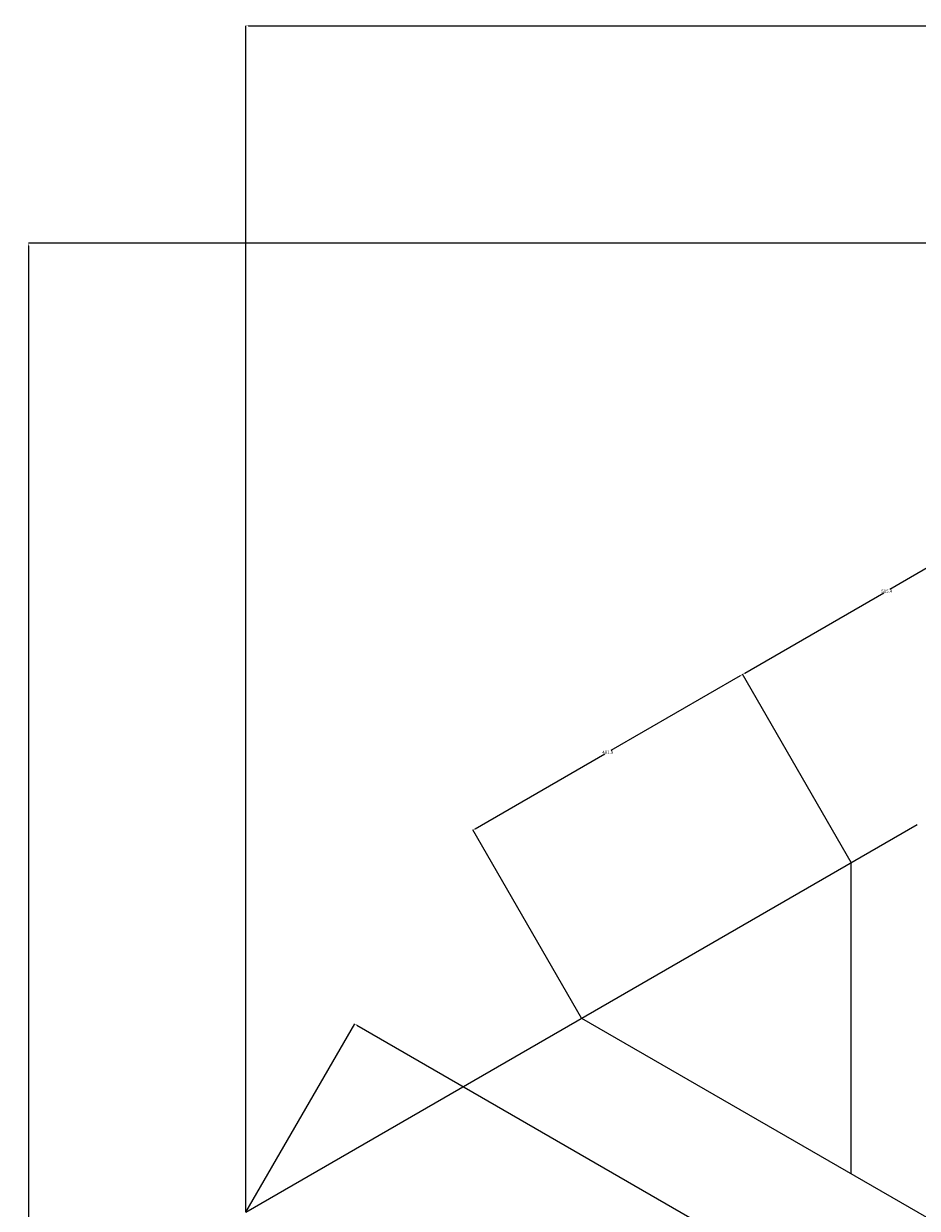
# Model space of a CAD drawing. Units: metres. Extents: x -2391 to 4922, y -635 to 4845.
# Tile 19 of 37: x -2391 to -1008, y 3011 to 4845. Entities that reach past the tile are written whole.
import ezdxf

# ---------------------------------------------------------------- set-up
doc = ezdxf.new("R2010")
doc.units = ezdxf.units.M
doc.header["$MEASUREMENT"] = 0
doc.layers.add('A-ANNO-DIMS', color=2, linetype='Continuous', lineweight=18)
doc.layers.add('A-FLOR-FIXT', color=3, linetype='Continuous', lineweight=25)
doc.styles.get("Standard").update_dxf_attribs({"font": 'arial.ttf'})
doc.dimstyles.get("Standard").update_dxf_attribs({"dimtxt": 5, "dimasz": 4, "dimexe": 0.18, "dimexo": 0.0625, "dimgap": 0.09, "dimtad": 0, "dimtih": 1, "dimtoh": 1, "dimdec": 0, "dimzin": 0, "dimdsep": 46, "dimtxsty": 'Standard', "dimcen": 0.09, "dimadec": 0, "dimazin": 0, "dimtfac": 1, "dimtdec": 0, "dimtofl": 0, "dimtmove": 0, "dimatfit": 3, "dimfxl": 1, "dimtolj": 1, "dimtzin": 0, "dimarcsym": 0})

# ---------------------------------------------------------------- blocks, each defined once
blk = doc.blocks.new('*D9')
at = {"layer": 'A-ANNO-DIMS', "color": 0, "lineweight": -2, "transparency": 16777216}
for p, q in [((-2047.3, 3005.3), (-2047.3, 4842)), ((-2043.3, 4841.8), (-755.9, 4841.8)), ((546.7, 4841.8), (-740.7, 4841.8)), ((550.7, 4505.3), (550.7, 4842))]:
    blk.add_line(p, q, dxfattribs=at)
at = {"layer": 'A-ANNO-DIMS', "color": 0, "transparency": 16777216}
for points in [[(-2043.3, 4842.4), (-2043.3, 4841.1), (-2047.3, 4841.8)], [(546.7, 4842.4), (546.7, 4841.1), (550.7, 4841.8)]]:
    blk.add_solid(points, dxfattribs=at)
at = {"layer": 'Defpoints', "color": 0, "transparency": 16777216}
for p in [(550.7, 4841.8), (550.7, 4505.3), (-2047.3, 3005.3)]:
    blk.add_point(p, dxfattribs=at)
at = {"layer": 'A-ANNO-DIMS', "color": 0, "transparency": 16777216, "insert": (-748.3, 4841.8), "char_height": 5, "attachment_point": 5}
blk.add_mtext('\\A1;2598', dxfattribs=at)
blk = doc.blocks.new('*D10')
at = {"layer": 'A-ANNO-DIMS', "color": 0, "lineweight": -2, "transparency": 16777216}
for p, q in [((550.7, 4505.3), (-2384, 4505.3)), ((-2383.8, 4501.3), (-2383.8, 2107.9)), ((-2383.8, -290.7), (-2383.8, 2102.6)), ((-488.6, -294.7), (-2384, -294.7))]:
    blk.add_line(p, q, dxfattribs=at)
at = {"layer": 'A-ANNO-DIMS', "color": 0, "transparency": 16777216}
for points in [[(-2384.5, 4501.3), (-2383.2, 4501.3), (-2383.8, 4505.3)], [(-2384.5, -290.7), (-2383.2, -290.7), (-2383.8, -294.7)]]:
    blk.add_solid(points, dxfattribs=at)
at = {"layer": 'Defpoints', "color": 0, "transparency": 16777216}
for p in [(-2383.8, 4505.3), (550.7, 4505.3), (-488.5, -294.7)]:
    blk.add_point(p, dxfattribs=at)
at = {"layer": 'A-ANNO-DIMS', "color": 0, "transparency": 16777216, "insert": (-2383.8, 2105.3), "char_height": 5, "attachment_point": 5}
blk.add_mtext('\\A1;4800', dxfattribs=at)
blk = doc.blocks.new('*D36')
at = {"layer": 'A-ANNO-DIMS', "color": 0, "lineweight": -2, "transparency": 16777216}
for p, q in [((-1282.1, 3835.7), (-1482.7, 3719.8)), ((-1110.4, 3546.3), (-1278.7, 3837.8)), ((-1692.5, 3598.7), (-1491.9, 3714.5)), ((-1527.8, 3305.3), (-1696.1, 3596.8))]:
    blk.add_line(p, q, dxfattribs=at)
at = {"layer": 'A-ANNO-DIMS', "color": 0, "transparency": 16777216}
for points in [[(-1282.4, 3836.2), (-1281.7, 3835.1), (-1278.6, 3837.7)], [(-1692.8, 3599.3), (-1692.2, 3598.1), (-1696, 3596.7)]]:
    blk.add_solid(points, dxfattribs=at)
at = {"layer": 'Defpoints', "color": 0, "transparency": 16777216}
for p in [(-1278.6, 3837.7), (-1110.4, 3546.2), (-1527.7, 3305.3)]:
    blk.add_point(p, dxfattribs=at)
at = {"layer": 'A-ANNO-DIMS', "color": 0, "transparency": 16777216, "insert": (-1487.3, 3717.2), "char_height": 5, "attachment_point": 5}
blk.add_mtext('\\A1;481.9', dxfattribs=at)
blk = doc.blocks.new('*D37')
at = {"layer": 'A-ANNO-DIMS', "color": 0, "lineweight": -2, "transparency": 16777216}
for p, q in [((-835.7, 4093.4), (-1050.8, 3969.2)), ((-664, 3804), (-832.3, 4095.5)), ((-1275.1, 3839.7), (-1060, 3963.9)), ((-1110.4, 3546.3), (-1278.7, 3837.8))]:
    blk.add_line(p, q, dxfattribs=at)
at = {"layer": 'A-ANNO-DIMS', "color": 0, "transparency": 16777216}
for points in [[(-836, 4094), (-835.4, 4092.8), (-832.2, 4095.4)], [(-1275.5, 3840.2), (-1274.8, 3839.1), (-1278.6, 3837.7)]]:
    blk.add_solid(points, dxfattribs=at)
at = {"layer": 'Defpoints', "color": 0, "transparency": 16777216}
for p in [(-832.2, 4095.4), (-664, 3804), (-1110.4, 3546.2)]:
    blk.add_point(p, dxfattribs=at)
at = {"layer": 'A-ANNO-DIMS', "color": 0, "transparency": 16777216, "insert": (-1055.4, 3966.5), "char_height": 5, "attachment_point": 5}
blk.add_mtext('\\A1;515.4', dxfattribs=at)
blk = doc.blocks.new('*D41')
at = {"layer": 'A-ANNO-DIMS', "color": 0, "lineweight": -2, "transparency": 16777216}
for p, q in [((-2047.3, 3005.3), (-1879, 3296.8)), ((-1875.6, 3294.7), (-1104.2, 2849.3)), ((-323.7, 2398.7), (-1095.1, 2844.1)), ((-488.5, 2105.3), (-320.1, 2396.8))]:
    blk.add_line(p, q, dxfattribs=at)
at = {"layer": 'A-ANNO-DIMS', "color": 0, "transparency": 16777216}
for points in [[(-1875.3, 3295.3), (-1876, 3294.1), (-1879.1, 3296.7)], [(-323.4, 2399.3), (-324, 2398.1), (-320.2, 2396.7)]]:
    blk.add_solid(points, dxfattribs=at)
at = {"layer": 'Defpoints', "color": 0, "transparency": 16777216}
for p in [(-2047.3, 3005.3), (-320.2, 2396.7), (-488.5, 2105.3)]:
    blk.add_point(p, dxfattribs=at)
at = {"layer": 'A-ANNO-DIMS', "color": 0, "transparency": 16777216, "insert": (-1099.7, 2846.7), "char_height": 5, "attachment_point": 5}
blk.add_mtext('\\A1;1800', dxfattribs=at)

msp = doc.modelspace()

# ---------------------------------------------------------------- linework, layer by layer
at = {"layer": 'A-FLOR-FIXT'}
for p, q in [((-2047.3343, 3005.2763), (-1008.1038, 3605.2763)), ((-1110.3549, 3064.311), (-1110.3549, 3546.2416)), ((-1527.7191, 3305.2763), (31.1266, 2405.2763))]:
    msp.add_line(p, q, dxfattribs=at)

# ---------------------------------------------------------------- dimensions: what is measured, and where the dimension line sits
at = {"layer": 'A-ANNO-DIMS'}
dim = msp.add_linear_dim(base=(550.7419, 4841.7763), p1=(-2047.3343, 3005.2763), p2=(550.7419, 4505.2763), dimstyle='Standard', override={"dimdec": 0, "dimlfac": 1, "dimrnd": 0, "dimzin": 0, "dimdsep": 46, "dimlunit": 2}, dxfattribs=at)
dim.commit()
dim.dimension.update_dxf_attribs({"geometry": '*D9', "text_midpoint": (-748.2962, 4841.7763)})
for base, p1, p2, angle, override, picture, middle in [((-2383.8343, 4505.2763), (-488.4886, -294.7237), (550.7419, 4505.2763), 90, {"dimdec": 0, "dimlfac": 1, "dimrnd": 0, "dimzin": 0, "dimdsep": 46, "dimlunit": 2}, '*D10', (-2383.8343, 2105.2763)), ((-832.2242, 4095.3771), (-1110.3549, 3546.2416), (-663.9742, 3803.9596), 30, {"dimdec": 1, "dimlfac": 1, "dimrnd": 0, "dimzin": 0, "dimdsep": 46, "dimlunit": 2}, '*D37', (-1055.4146, 3966.5181)), ((-1278.6049, 3837.6591), (-1527.7191, 3305.2763), (-1110.3549, 3546.2416), 30, {"dimdec": 1, "dimlfac": 1, "dimrnd": 0, "dimzin": 0, "dimdsep": 46, "dimlunit": 2}, '*D36', (-1487.287, 3717.1765)), ((-320.2386, 2396.6938), (-2047.3343, 3005.2763), (-488.4886, 2105.2763), 330, {"dimdec": 0, "dimlfac": 1, "dimrnd": 0, "dimzin": 0, "dimdsep": 46, "dimlunit": 2}, '*D41', (-1099.6615, 2846.6938))]:
    dim = msp.add_linear_dim(base=base, p1=p1, p2=p2, angle=angle, dimstyle='Standard', override=override, dxfattribs=at)
    dim.commit()
    dim.dimension.update_dxf_attribs({"geometry": picture, "text_midpoint": middle})

doc.saveas('drawing.dxf')
